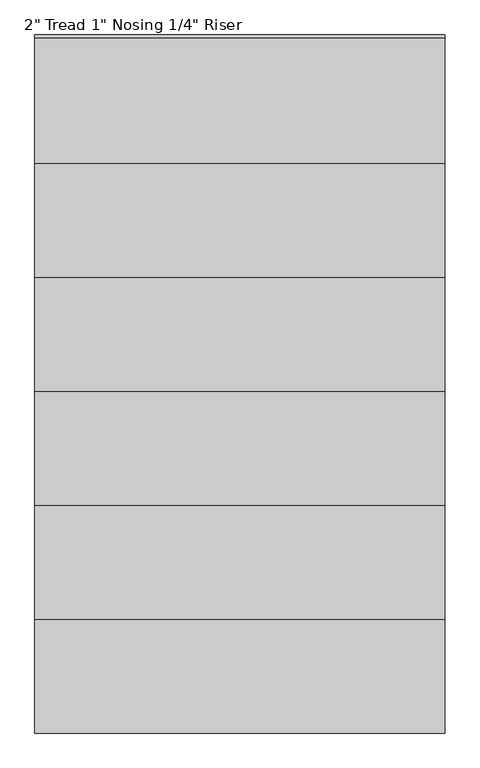
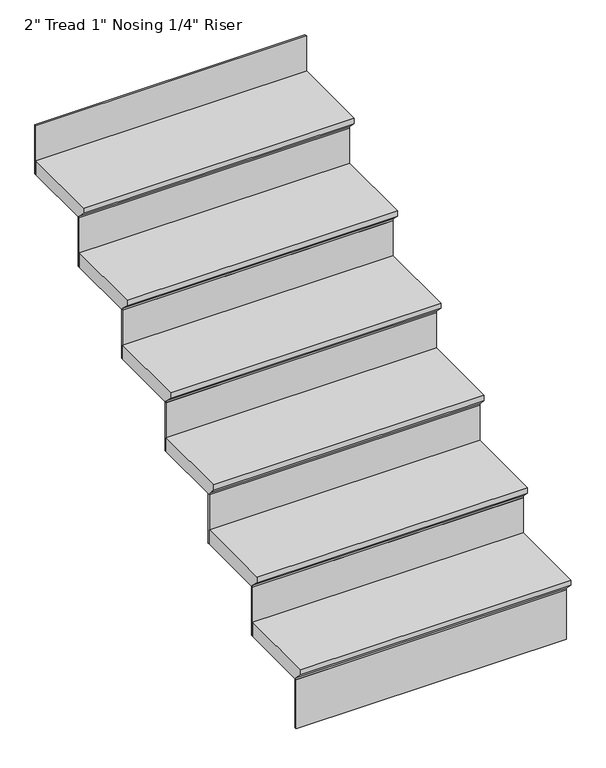
"""IFC4 building model written with IfcOpenShell, lengths in millimetres: stair flight geometry."""

from ifc_helpers import new_model, si_unit, frame, origin, place, context, project, spatial, polyline, outline, extrude, source, transform, mapped, element, save


def stair_flight_de56df94(model_context):
    return source(origin(), model_context, "Body", "SweptSolid", [
        extrude(outline(polyline([(-4867.8688563, 1230.9230769), (-4588.4688563, 1230.9230769), (-4588.4688563, 1180.1230769), (-4842.4688563, 1180.1230769), (-4842.4688563, 1186.4730769), (-4867.8688563, 1211.8730769), (-4867.8688563, 1230.9230769)])), frame((-5540.3879317, 0.0, 0.0), z_axis=(1.0, 0.0, 0.0), x_axis=(0.0, 1.0, 0.0)), (0.0, 0.0, 1.0), 914.4),
        extrude(outline(polyline([(-4625.9879317, -4836.1188563), (-4625.9879317, -4842.4688563), (-5540.3879317, -4842.4688563), (-5540.3879317, -4836.1188563), (-4625.9879317, -4836.1188563)])), frame((0.0, 0.0, 1004.2769231), z_axis=(0.0, 0.0, 1.0), x_axis=(1.0, 0.0, 0.0)), (0.0, 0.0, 1.0), 175.8461538),
        extrude(outline(polyline([(-4625.9879317, -4582.1188563), (-4625.9879317, -4588.4688563), (-5540.3879317, -4588.4688563), (-5540.3879317, -4582.1188563), (-4625.9879317, -4582.1188563)])), frame((0.0, 0.0, 1180.1230769), z_axis=(0.0, 0.0, 1.0), x_axis=(1.0, 0.0, 0.0)), (0.0, 0.0, 1.0), 175.8461538),
        extrude(outline(polyline([(-4613.8688563, 1406.7692308), (-4334.4688563, 1406.7692308), (-4334.4688563, 1355.9692308), (-4588.4688563, 1355.9692308), (-4588.4688563, 1362.3192308), (-4613.8688563, 1387.7192308), (-4613.8688563, 1406.7692308)])), frame((-5540.3879317, 0.0, 0.0), z_axis=(1.0, 0.0, 0.0), x_axis=(0.0, 1.0, 0.0)), (0.0, 0.0, 1.0), 914.4),
        extrude(outline(polyline([(-4625.9879317, -4328.1188563), (-4625.9879317, -4334.4688563), (-5540.3879317, -4334.4688563), (-5540.3879317, -4328.1188563), (-4625.9879317, -4328.1188563)])), frame((0.0, 0.0, 1355.9692308), z_axis=(0.0, 0.0, 1.0), x_axis=(1.0, 0.0, 0.0)), (0.0, 0.0, 1.0), 175.8461538),
        extrude(outline(polyline([(-4359.8688563, 1582.6153846), (-4080.4688563, 1582.6153846), (-4080.4688563, 1531.8153846), (-4334.4688563, 1531.8153846), (-4334.4688563, 1538.1653846), (-4359.8688563, 1563.5653846), (-4359.8688563, 1582.6153846)])), frame((-5540.3879317, 0.0, 0.0), z_axis=(1.0, 0.0, 0.0), x_axis=(0.0, 1.0, 0.0)), (0.0, 0.0, 1.0), 914.4),
        extrude(outline(polyline([(-4625.9879317, -4074.1188563), (-4625.9879317, -4080.4688563), (-5540.3879317, -4080.4688563), (-5540.3879317, -4074.1188563), (-4625.9879317, -4074.1188563)])), frame((0.0, 0.0, 1531.8153846), z_axis=(0.0, 0.0, 1.0), x_axis=(1.0, 0.0, 0.0)), (0.0, 0.0, 1.0), 175.8461538),
        extrude(outline(polyline([(-4105.8688563, 1758.4615385), (-3826.4688563, 1758.4615385), (-3826.4688563, 1707.6615385), (-4080.4688563, 1707.6615385), (-4080.4688563, 1714.0115385), (-4105.8688563, 1739.4115385), (-4105.8688563, 1758.4615385)])), frame((-5540.3879317, 0.0, 0.0), z_axis=(1.0, 0.0, 0.0), x_axis=(0.0, 1.0, 0.0)), (0.0, 0.0, 1.0), 914.4),
        extrude(outline(polyline([(-4625.9879317, -3820.1188563), (-4625.9879317, -3826.4688563), (-5540.3879317, -3826.4688563), (-5540.3879317, -3820.1188563), (-4625.9879317, -3820.1188563)])), frame((0.0, 0.0, 1707.6615385), z_axis=(0.0, 0.0, 1.0), x_axis=(1.0, 0.0, 0.0)), (0.0, 0.0, 1.0), 175.8461538),
        extrude(outline(polyline([(-3851.8688563, 1934.3076923), (-3572.4688563, 1934.3076923), (-3572.4688563, 1883.5076923), (-3826.4688563, 1883.5076923), (-3826.4688563, 1889.8576923), (-3851.8688563, 1915.2576923), (-3851.8688563, 1934.3076923)])), frame((-5540.3879317, 0.0, 0.0), z_axis=(1.0, 0.0, 0.0), x_axis=(0.0, 1.0, 0.0)), (0.0, 0.0, 1.0), 914.4),
        extrude(outline(polyline([(-4625.9879317, -3566.1188563), (-4625.9879317, -3572.4688563), (-5540.3879317, -3572.4688563), (-5540.3879317, -3566.1188563), (-4625.9879317, -3566.1188563)])), frame((0.0, 0.0, 1883.5076923), z_axis=(0.0, 0.0, 1.0), x_axis=(1.0, 0.0, 0.0)), (0.0, 0.0, 1.0), 175.8461538),
        extrude(outline(polyline([(-4625.9879317, -3312.1188563), (-4625.9879317, -3318.4688563), (-5540.3879317, -3318.4688563), (-5540.3879317, -3312.1188563), (-4625.9879317, -3312.1188563)])), frame((0.0, 0.0, 2059.3538462), z_axis=(0.0, 0.0, 1.0), x_axis=(1.0, 0.0, 0.0)), (0.0, 0.0, 1.0), 175.8461538),
        extrude(outline(polyline([(-3597.8688563, 2110.1538462), (-3318.4688563, 2110.1538462), (-3318.4688563, 2059.3538462), (-3572.4688563, 2059.3538462), (-3572.4688563, 2065.7038462), (-3597.8688563, 2091.1038462), (-3597.8688563, 2110.1538462)])), frame((-5540.3879317, 0.0, 0.0), z_axis=(1.0, 0.0, 0.0), x_axis=(0.0, 1.0, 0.0)), (0.0, 0.0, 1.0), 914.4),
    ])


if __name__ == "__main__":
    model = new_model("IFC4")
    model_context = context("Model", 3, world=origin())
    ifc_project = project(units=[si_unit("LENGTHUNIT", "METRE", prefix="MILLI")], contexts=[model_context])
    site = spatial("IfcSite", under=ifc_project)
    building = spatial("IfcBuilding", under=site)
    placement = place(None, origin())
    stair_flight_shape = stair_flight_de56df94(model_context)
    element("IfcStairFlight", 1, ObjectType="2\" Tread 1\" Nosing 1/4\" Riser", at=placement, inside=building, context=model_context, shape_type="MappedRepresentation", body=[
        mapped(stair_flight_shape, transform((0.0, 0.0, 0.0), x_axis=(1.0, 0.0, 0.0), y_axis=(0.0, 1.0, 0.0), z_axis=(0.0, 0.0, 1.0))),
    ])
    save(model, "model.ifc")
